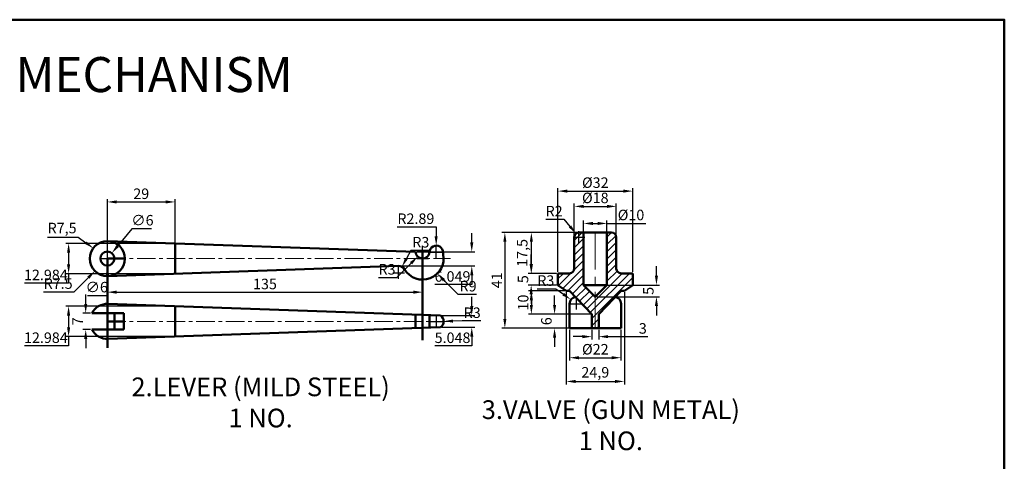
# Model space of a CAD drawing. Units: millimetres. Extents: x -166 to 681, y -4360 to 126.
# Tile 7 of 7: x 259 to 681, y -63 to 126. Entities that reach past the tile are written whole.
import ezdxf

# ---------------------------------------------------------------- set-up
doc = ezdxf.new("R2010")
doc.units = ezdxf.units.MM
doc.header["$LTSCALE"] = 0.5
doc.linetypes.add('CENTER', pattern=[50.8, 31.75, -6.35, 6.35, -6.35])
for name, color, linetype, lineweight in [('M-CNTR', 1, 'CENTER', 18), ('M-DIMS', 2, 'Continuous', 25), ('M-HATC', 8, 'Continuous', 18), ('M-OUTL', 7, 'Continuous', 50), ('M-TEXT', 7, 'Continuous', 25), ('M-TTLB', 7, 'Continuous', 50)]:
    doc.layers.add(name, color=color, linetype=linetype, lineweight=lineweight)
doc.styles.get("Standard").update_dxf_attribs({"font": 'arial.ttf'})
doc.dimstyles.new('ISO-25', dxfattribs={"dimtxt": 4.5, "dimasz": 4, "dimexe": 1.25, "dimexo": 0.625, "dimtad": 1, "dimtoh": 1, "dimdec": 1, "dimtxsty": 'Standard', "dimcen": 2.5, "dimadec": 0, "dimazin": 0, "dimtfac": 1, "dimtdec": 1, "dimtofl": 0, "dimtmove": 0, "dimatfit": 3, "dimfxl": 1, "dimarcsym": 0})

# ---------------------------------------------------------------- blocks, each defined once
blk = doc.blocks.new('*D25')
at = {"layer": 'Defpoints', "color": 0, "ltscale": 0.5, "transparency": 16777216}
for p in [(521.63, 52.7), (489.63, 17.51), (521.63, 17.51)]:
    blk.add_point(p, dxfattribs=at)
at = {"layer": 'M-DIMS', "color": 0, "lineweight": -2, "ltscale": 0.5, "transparency": 16777216}
for p, q in [((489.63, 18.13), (489.63, 53.95)), ((493.63, 52.7), (517.63, 52.7)), ((521.63, 18.13), (521.63, 53.95))]:
    blk.add_line(p, q, dxfattribs=at)
at = {"layer": 'M-DIMS', "color": 0, "ltscale": 0.5, "transparency": 16777216}
for points in [[(493.63, 53.37), (493.63, 52.04), (489.63, 52.7)], [(517.63, 53.37), (517.63, 52.04), (521.63, 52.7)]]:
    blk.add_solid(points, dxfattribs=at)
at = {"layer": 'M-DIMS', "color": 0, "ltscale": 0.5, "transparency": 16777216, "insert": (505.63, 55.75), "char_height": 4.5, "attachment_point": 5}
blk.add_mtext('%%C32', dxfattribs=at)
blk = doc.blocks.new('*D26')
at = {"layer": 'Defpoints', "color": 0, "ltscale": 0.5, "transparency": 16777216}
for p in [(510.63, 38.86), (500.63, 35.01), (510.63, 35.01)]:
    blk.add_point(p, dxfattribs=at)
at = {"layer": 'M-DIMS', "color": 0, "lineweight": -2, "ltscale": 0.5, "transparency": 16777216}
for p, q in [((500.63, 35.63), (500.63, 40.11)), ((504.63, 38.86), (506.63, 38.86)), ((510.63, 35.63), (510.63, 40.11)), ((510.63, 38.86), (527.21, 38.86))]:
    blk.add_line(p, q, dxfattribs=at)
at = {"layer": 'M-DIMS', "color": 0, "ltscale": 0.5, "transparency": 16777216}
for points in [[(504.63, 39.53), (504.63, 38.19), (500.63, 38.86)], [(506.63, 39.53), (506.63, 38.19), (510.63, 38.86)]]:
    blk.add_solid(points, dxfattribs=at)
at = {"layer": 'M-DIMS', "color": 0, "ltscale": 0.5, "transparency": 16777216, "insert": (520.92, 41.91), "char_height": 4.5, "attachment_point": 5}
blk.add_mtext('%%C10', dxfattribs=at)
blk = doc.blocks.new('*D27')
at = {"layer": 'Defpoints', "color": 0, "ltscale": 0.5, "transparency": 16777216}
for p in [(514.63, 46.17), (496.63, 26.26), (514.63, 26.26)]:
    blk.add_point(p, dxfattribs=at)
at = {"layer": 'M-DIMS', "color": 0, "lineweight": -2, "ltscale": 0.5, "transparency": 16777216}
for p, q in [((496.63, 26.88), (496.63, 47.42)), ((514.63, 26.88), (514.63, 47.42)), ((500.63, 46.17), (510.63, 46.17))]:
    blk.add_line(p, q, dxfattribs=at)
at = {"layer": 'M-DIMS', "color": 0, "ltscale": 0.5, "transparency": 16777216}
for points in [[(500.63, 46.84), (500.63, 45.51), (496.63, 46.17)], [(510.63, 46.84), (510.63, 45.51), (514.63, 46.17)]]:
    blk.add_solid(points, dxfattribs=at)
at = {"layer": 'M-DIMS', "color": 0, "ltscale": 0.5, "transparency": 16777216, "insert": (505.63, 49.22), "char_height": 4.5, "attachment_point": 5}
blk.add_mtext('%%C18', dxfattribs=at)
blk = doc.blocks.new('*D28')
at = {"layer": 'Defpoints', "color": 0, "ltscale": 0.5, "transparency": 16777216}
for p in [(505.63, 12.51), (505.63, 7.51), (531.82, 7.51)]:
    blk.add_point(p, dxfattribs=at)
at = {"layer": 'M-DIMS', "color": 0, "lineweight": -2, "ltscale": 0.5, "transparency": 16777216}
for p, q in [((531.82, 16.51), (531.82, 20.51)), ((506.26, 12.51), (533.07, 12.51)), ((506.26, 7.51), (533.07, 7.51)), ((531.82, 3.51), (531.82, -0.49))]:
    blk.add_line(p, q, dxfattribs=at)
at = {"layer": 'M-DIMS', "color": 0, "ltscale": 0.5, "transparency": 16777216}
for points in [[(531.15, 16.51), (532.49, 16.51), (531.82, 12.51)], [(531.15, 3.51), (532.49, 3.51), (531.82, 7.51)]]:
    blk.add_solid(points, dxfattribs=at)
at = {"layer": 'M-DIMS', "color": 0, "ltscale": 0.5, "transparency": 16777216, "insert": (528.91, 10.01), "char_height": 4.5, "attachment_point": 5, "rotation": 90}
blk.add_mtext('5', dxfattribs=at)
blk = doc.blocks.new('*D29')
at = {"layer": 'Defpoints', "color": 0, "ltscale": 0.5, "transparency": 16777216}
for p in [(505.63, 35.01), (466.89, -5.99), (505.63, -5.99)]:
    blk.add_point(p, dxfattribs=at)
at = {"layer": 'M-DIMS', "color": 0, "lineweight": -2, "ltscale": 0.5, "transparency": 16777216}
for p, q in [((505.01, 35.01), (465.64, 35.01)), ((466.89, 31.01), (466.89, -1.99)), ((505.01, -5.99), (465.64, -5.99))]:
    blk.add_line(p, q, dxfattribs=at)
at = {"layer": 'M-DIMS', "color": 0, "ltscale": 0.5, "transparency": 16777216}
for points in [[(466.23, 31.01), (467.56, 31.01), (466.89, 35.01)], [(466.23, -1.99), (467.56, -1.99), (466.89, -5.99)]]:
    blk.add_solid(points, dxfattribs=at)
at = {"layer": 'M-DIMS', "color": 0, "ltscale": 0.5, "transparency": 16777216, "insert": (464.01, 14.51), "char_height": 4.5, "attachment_point": 5, "rotation": 90}
blk.add_mtext('41', dxfattribs=at)
blk = doc.blocks.new('*D30')
at = {"layer": 'Defpoints', "color": 0, "ltscale": 0.5, "transparency": 16777216}
for p in [(478.25, 35.01), (485.33, 35.01), (489.63, 17.51)]:
    blk.add_point(p, dxfattribs=at)
at = {"layer": 'M-DIMS', "color": 0, "lineweight": -2, "ltscale": 0.5, "transparency": 16777216}
for p, q in [((484.7, 35.01), (477, 35.01)), ((478.25, 21.51), (478.25, 31.01)), ((489.01, 17.51), (477, 17.51))]:
    blk.add_line(p, q, dxfattribs=at)
at = {"layer": 'M-DIMS', "color": 0, "ltscale": 0.5, "transparency": 16777216}
for points in [[(477.58, 31.01), (478.91, 31.01), (478.25, 35.01)], [(477.58, 21.51), (478.91, 21.51), (478.25, 17.51)]]:
    blk.add_solid(points, dxfattribs=at)
at = {"layer": 'M-DIMS', "color": 0, "ltscale": 0.5, "transparency": 16777216, "insert": (474.92, 26.26), "char_height": 4.5, "attachment_point": 5, "rotation": 90}
blk.add_mtext('17,5', dxfattribs=at)
blk = doc.blocks.new('*D31')
at = {"layer": 'Defpoints', "color": 0, "ltscale": 0.5, "transparency": 16777216}
for p in [(493.19, 10.01), (478.25, 0.01), (504.13, 0.01)]:
    blk.add_point(p, dxfattribs=at)
at = {"layer": 'M-DIMS', "color": 0, "lineweight": -2, "ltscale": 0.5, "transparency": 16777216}
for p, q in [((492.57, 10.01), (477, 10.01)), ((478.25, 6.01), (478.25, 4.01)), ((503.51, 0.01), (477, 0.01))]:
    blk.add_line(p, q, dxfattribs=at)
at = {"layer": 'M-DIMS', "color": 0, "ltscale": 0.5, "transparency": 16777216}
for points in [[(477.58, 6.01), (478.91, 6.01), (478.25, 10.01)], [(477.58, 4.01), (478.91, 4.01), (478.25, 0.01)]]:
    blk.add_solid(points, dxfattribs=at)
at = {"layer": 'M-DIMS', "color": 0, "ltscale": 0.5, "transparency": 16777216, "insert": (475.32, 5.01), "char_height": 4.5, "attachment_point": 5, "rotation": 90}
blk.add_mtext('10', dxfattribs=at)
blk = doc.blocks.new('*D32')
at = {"layer": 'Defpoints', "color": 0, "ltscale": 0.5, "transparency": 16777216}
for p in [(504.13, 0.01), (488.18, -5.99), (504.13, -5.99)]:
    blk.add_point(p, dxfattribs=at)
at = {"layer": 'M-DIMS', "color": 0, "lineweight": -2, "ltscale": 0.5, "transparency": 16777216}
for p, q in [((488.18, 4.01), (488.18, 8.01)), ((503.51, 0.01), (486.93, 0.01)), ((503.51, -5.99), (486.93, -5.99)), ((488.18, -9.99), (488.18, -13.99))]:
    blk.add_line(p, q, dxfattribs=at)
at = {"layer": 'M-DIMS', "color": 0, "ltscale": 0.5, "transparency": 16777216}
for points in [[(487.52, 4.01), (488.85, 4.01), (488.18, 0.01)], [(487.52, -9.99), (488.85, -9.99), (488.18, -5.99)]]:
    blk.add_solid(points, dxfattribs=at)
at = {"layer": 'M-DIMS', "color": 0, "ltscale": 0.5, "transparency": 16777216, "insert": (485.26, -2.99), "char_height": 4.5, "attachment_point": 5, "rotation": 90}
blk.add_mtext('6', dxfattribs=at)
blk = doc.blocks.new('*D33')
at = {"layer": 'Defpoints', "color": 0, "ltscale": 0.5, "transparency": 16777216}
for p in [(489.63, 17.51), (478.15, 12.51), (489.63, 12.51)]:
    blk.add_point(p, dxfattribs=at)
at = {"layer": 'M-DIMS', "color": 0, "lineweight": -2, "ltscale": 0.5, "transparency": 16777216}
for p, q in [((478.15, 21.51), (478.15, 25.51)), ((489.01, 17.51), (476.9, 17.51)), ((489.01, 12.51), (476.9, 12.51)), ((478.15, 8.51), (478.15, 4.51))]:
    blk.add_line(p, q, dxfattribs=at)
at = {"layer": 'M-DIMS', "color": 0, "ltscale": 0.5, "transparency": 16777216}
for points in [[(477.48, 21.51), (478.82, 21.51), (478.15, 17.51)], [(477.48, 8.51), (478.82, 8.51), (478.15, 12.51)]]:
    blk.add_solid(points, dxfattribs=at)
at = {"layer": 'M-DIMS', "color": 0, "ltscale": 0.5, "transparency": 16777216, "insert": (475.24, 15.01), "char_height": 4.5, "attachment_point": 5, "rotation": 90}
blk.add_mtext('5', dxfattribs=at)
blk = doc.blocks.new('*D34')
at = {"layer": 'Defpoints', "color": 0, "ltscale": 0.5, "transparency": 16777216}
for p in [(504.13, -5.99), (507.13, -5.99), (507.13, -9.59)]:
    blk.add_point(p, dxfattribs=at)
at = {"layer": 'M-DIMS', "color": 0, "lineweight": -2, "ltscale": 0.5, "transparency": 16777216}
for p, q in [((504.13, -6.62), (504.13, -10.84)), ((507.13, -6.62), (507.13, -10.84)), ((500.13, -9.59), (496.13, -9.59)), ((511.13, -9.59), (528.08, -9.59))]:
    blk.add_line(p, q, dxfattribs=at)
at = {"layer": 'M-DIMS', "color": 0, "ltscale": 0.5, "transparency": 16777216}
for points in [[(500.13, -8.92), (500.13, -10.25), (504.13, -9.59)], [(511.13, -8.92), (511.13, -10.25), (507.13, -9.59)]]:
    blk.add_solid(points, dxfattribs=at)
at = {"layer": 'M-DIMS', "color": 0, "ltscale": 0.5, "transparency": 16777216, "insert": (525.98, -6.66), "char_height": 4.5, "attachment_point": 5}
blk.add_mtext('3', dxfattribs=at)
blk = doc.blocks.new('*D35')
at = {"layer": 'Defpoints', "color": 0, "ltscale": 0.5, "transparency": 16777216}
for p in [(494.63, -5.99), (516.63, -5.99), (516.63, -18.62)]:
    blk.add_point(p, dxfattribs=at)
at = {"layer": 'M-DIMS', "color": 0, "lineweight": -2, "ltscale": 0.5, "transparency": 16777216}
for p, q in [((494.63, -6.62), (494.63, -19.87)), ((516.63, -6.62), (516.63, -19.87)), ((498.63, -18.62), (512.63, -18.62))]:
    blk.add_line(p, q, dxfattribs=at)
at = {"layer": 'M-DIMS', "color": 0, "ltscale": 0.5, "transparency": 16777216}
for points in [[(498.63, -17.95), (498.63, -19.29), (494.63, -18.62)], [(512.63, -17.95), (512.63, -19.29), (516.63, -18.62)]]:
    blk.add_solid(points, dxfattribs=at)
at = {"layer": 'M-DIMS', "color": 0, "ltscale": 0.5, "transparency": 16777216, "insert": (505.63, -15.57), "char_height": 4.5, "attachment_point": 5}
blk.add_mtext('%%C22', dxfattribs=at)
blk = doc.blocks.new('*D36')
at = {"layer": 'Defpoints', "color": 0, "ltscale": 0.5, "transparency": 16777216}
for p in [(493.19, 10.01), (518.08, 10.01), (518.08, -28.77)]:
    blk.add_point(p, dxfattribs=at)
at = {"layer": 'M-DIMS', "color": 0, "lineweight": -2, "ltscale": 0.5, "transparency": 16777216}
for p, q in [((493.19, 9.38), (493.19, -30.02)), ((518.08, 9.38), (518.08, -30.02)), ((497.19, -28.77), (514.08, -28.77))]:
    blk.add_line(p, q, dxfattribs=at)
at = {"layer": 'M-DIMS', "color": 0, "ltscale": 0.5, "transparency": 16777216}
for points in [[(497.19, -28.11), (497.19, -29.44), (493.19, -28.77)], [(514.08, -28.11), (514.08, -29.44), (518.08, -28.77)]]:
    blk.add_solid(points, dxfattribs=at)
at = {"layer": 'M-DIMS', "color": 0, "ltscale": 0.5, "transparency": 16777216, "insert": (505.63, -25.44), "char_height": 4.5, "attachment_point": 5}
blk.add_mtext('24,9', dxfattribs=at)
blk = doc.blocks.new('*D69')
at = {"layer": 'Defpoints', "color": 0, "ltscale": 0.5, "transparency": 16777216}
for p in [(298.56, 26.14), (294.76, 21.5)]:
    blk.add_point(p, dxfattribs=at)
at = {"layer": 'M-DIMS', "color": 0, "lineweight": -2, "ltscale": 0.5, "transparency": 16777216}
for p, q in [((307.13, 36.61), (301.1, 29.24)), ((315.6, 36.61), (307.13, 36.61)), ((296.66, 21.32), (296.66, 26.32)), ((294.16, 23.82), (299.16, 23.82))]:
    blk.add_line(p, q, dxfattribs=at)
at = {"layer": 'M-DIMS', "color": 0, "ltscale": 0.5, "transparency": 16777216}
blk.add_solid([(300.58, 29.66), (301.61, 28.82), (298.56, 26.14)], dxfattribs=at)
at = {"layer": 'M-DIMS', "color": 0, "ltscale": 0.5, "transparency": 16777216, "insert": (311.68, 39.66), "char_height": 4.5, "attachment_point": 5}
blk.add_mtext('∅6', dxfattribs=at)
blk = doc.blocks.new('*D70')
at = {"layer": 'Defpoints', "color": 0, "ltscale": 0.5, "transparency": 16777216}
for p in [(290.61, 28.26), (296.66, 23.82)]:
    blk.add_point(p, dxfattribs=at)
at = {"layer": 'M-DIMS', "color": 0, "lineweight": -2, "ltscale": 0.5, "transparency": 16777216}
for p, q in [((271.01, 33), (284.17, 33)), ((284.17, 33), (287.39, 30.63)), ((296.66, 21.32), (296.66, 26.32)), ((294.16, 23.82), (299.16, 23.82))]:
    blk.add_line(p, q, dxfattribs=at)
at = {"layer": 'M-DIMS', "color": 0, "ltscale": 0.5, "transparency": 16777216}
blk.add_solid([(287.78, 31.17), (287, 30.09), (290.61, 28.26)], dxfattribs=at)
at = {"layer": 'M-DIMS', "color": 0, "ltscale": 0.5, "transparency": 16777216, "insert": (277.27, 36.32), "char_height": 4.5, "attachment_point": 5}
blk.add_mtext('R7,5', dxfattribs=at)
blk = doc.blocks.new('*D71')
at = {"layer": 'Defpoints', "color": 0, "ltscale": 0.5, "transparency": 16777216}
for p in [(325.66, 48.07), (296.66, 23.82), (325.66, 23.82)]:
    blk.add_point(p, dxfattribs=at)
at = {"layer": 'M-DIMS', "color": 0, "lineweight": -2, "ltscale": 0.5, "transparency": 16777216}
for p, q in [((296.66, 24.45), (296.66, 49.32)), ((300.66, 48.07), (321.66, 48.07)), ((325.66, 24.45), (325.66, 49.32))]:
    blk.add_line(p, q, dxfattribs=at)
at = {"layer": 'M-DIMS', "color": 0, "ltscale": 0.5, "transparency": 16777216}
for points in [[(300.66, 48.74), (300.66, 47.4), (296.66, 48.07)], [(321.66, 48.74), (321.66, 47.4), (325.66, 48.07)]]:
    blk.add_solid(points, dxfattribs=at)
at = {"layer": 'M-DIMS', "color": 0, "ltscale": 0.5, "transparency": 16777216, "insert": (311.16, 50.99), "char_height": 4.5, "attachment_point": 5}
blk.add_mtext('29', dxfattribs=at)
blk = doc.blocks.new('*D72')
at = {"layer": 'Defpoints', "color": 0, "ltscale": 0.5, "transparency": 16777216}
for p in [(296.66, 10.75), (431.66, 10.75), (431.66, 9.45)]:
    blk.add_point(p, dxfattribs=at)
at = {"layer": 'M-DIMS', "color": 0, "lineweight": -2, "ltscale": 0.5, "transparency": 16777216}
for p, q in [((296.66, 10.12), (296.66, 8.2)), ((300.66, 9.45), (427.66, 9.45)), ((431.66, 10.12), (431.66, 8.2))]:
    blk.add_line(p, q, dxfattribs=at)
at = {"layer": 'M-DIMS', "color": 0, "ltscale": 0.5, "transparency": 16777216}
for points in [[(300.66, 10.12), (300.66, 8.79), (296.66, 9.45)], [(427.66, 10.12), (427.66, 8.79), (431.66, 9.45)]]:
    blk.add_solid(points, dxfattribs=at)
at = {"layer": 'M-DIMS', "color": 0, "ltscale": 0.5, "transparency": 16777216, "insert": (364.16, 12.38), "char_height": 4.5, "attachment_point": 5}
blk.add_mtext('135', dxfattribs=at)
blk = doc.blocks.new('*D73')
at = {"layer": 'Defpoints', "color": 0, "ltscale": 0.5, "transparency": 16777216}
for p in [(290.03, 0.45), (287.39, -6.55), (290.03, -6.55)]:
    blk.add_point(p, dxfattribs=at)
at = {"layer": 'M-DIMS', "color": 0, "lineweight": -2, "ltscale": 0.5, "transparency": 16777216}
for p, q in [((287.39, 4.45), (287.39, 8.45)), ((289.4, 0.45), (286.14, 0.45)), ((289.4, -6.55), (286.14, -6.55)), ((287.39, -10.55), (287.39, -14.55))]:
    blk.add_line(p, q, dxfattribs=at)
at = {"layer": 'M-DIMS', "color": 0, "ltscale": 0.5, "transparency": 16777216}
for points in [[(286.72, 4.45), (288.05, 4.45), (287.39, 0.45)], [(286.72, -10.55), (288.05, -10.55), (287.39, -6.55)]]:
    blk.add_solid(points, dxfattribs=at)
at = {"layer": 'M-DIMS', "color": 0, "ltscale": 0.5, "transparency": 16777216, "insert": (284.51, -3.05), "char_height": 4.5, "attachment_point": 5, "rotation": 90}
blk.add_mtext('7', dxfattribs=at)
blk = doc.blocks.new('*D83')
at = {"layer": 'Defpoints', "color": 0, "ltscale": 0.5, "transparency": 16777216}
for p in [(325.66, 30.32), (280.06, 17.33), (325.66, 17.33)]:
    blk.add_point(p, dxfattribs=at)
at = {"layer": 'M-DIMS', "color": 0, "lineweight": -2, "ltscale": 0.5, "transparency": 16777216}
for p, q in [((325.04, 30.32), (278.81, 30.32)), ((280.06, 26.32), (280.06, 21.33)), ((325.04, 17.33), (278.81, 17.33)), ((280.06, 17.33), (280.06, 13.33)), ((280.06, 13.33), (261.2, 13.33))]:
    blk.add_line(p, q, dxfattribs=at)
at = {"layer": 'M-DIMS', "color": 0, "ltscale": 0.5, "transparency": 16777216}
for points in [[(279.39, 26.32), (280.73, 26.32), (280.06, 30.32)], [(279.39, 21.33), (280.73, 21.33), (280.06, 17.33)]]:
    blk.add_solid(points, dxfattribs=at)
at = {"layer": 'M-DIMS', "color": 0, "ltscale": 0.5, "transparency": 16777216, "insert": (270.32, 16.25), "char_height": 4.5, "attachment_point": 5}
blk.add_mtext('12.984', dxfattribs=at)
blk = doc.blocks.new('*D84')
at = {"layer": 'Defpoints', "color": 0, "ltscale": 0.5, "transparency": 16777216}
for p in [(428.66, 26.72), (421.25, 20.67), (452.72, 20.67)]:
    blk.add_point(p, dxfattribs=at)
at = {"layer": 'M-DIMS', "color": 0, "lineweight": -2, "ltscale": 0.5, "transparency": 16777216}
for p, q in [((452.72, 30.72), (452.72, 34.72)), ((429.29, 26.72), (453.97, 26.72)), ((421.88, 20.67), (453.97, 20.67)), ((452.72, 12.67), (436.87, 12.67)), ((452.72, 16.67), (452.72, 12.67))]:
    blk.add_line(p, q, dxfattribs=at)
at = {"layer": 'M-DIMS', "color": 0, "ltscale": 0.5, "transparency": 16777216}
for points in [[(452.05, 30.72), (453.38, 30.72), (452.72, 26.72)], [(452.05, 16.67), (453.38, 16.67), (452.72, 20.67)]]:
    blk.add_solid(points, dxfattribs=at)
at = {"layer": 'M-DIMS', "color": 0, "ltscale": 0.5, "transparency": 16777216, "insert": (444.48, 15.59), "char_height": 4.5, "attachment_point": 5}
blk.add_mtext('6.049', dxfattribs=at)
blk = doc.blocks.new('*D85')
at = {"layer": 'Defpoints', "color": 0, "ltscale": 0.5, "transparency": 16777216}
for p in [(439.28, -0.53), (439.28, -5.58), (452.72, -5.58)]:
    blk.add_point(p, dxfattribs=at)
at = {"layer": 'M-DIMS', "color": 0, "lineweight": -2, "ltscale": 0.5, "transparency": 16777216}
for p, q in [((452.72, 3.47), (452.72, 7.47)), ((439.91, -0.53), (453.97, -0.53)), ((439.91, -5.58), (453.97, -5.58)), ((452.72, -9.58), (452.72, -13.58)), ((452.72, -13.58), (436.9, -13.58))]:
    blk.add_line(p, q, dxfattribs=at)
at = {"layer": 'M-DIMS', "color": 0, "ltscale": 0.5, "transparency": 16777216}
for points in [[(452.05, 3.47), (453.38, 3.47), (452.72, -0.53)], [(452.05, -9.58), (453.38, -9.58), (452.72, -5.58)]]:
    blk.add_solid(points, dxfattribs=at)
at = {"layer": 'M-DIMS', "color": 0, "ltscale": 0.5, "transparency": 16777216, "insert": (444.49, -10.65), "char_height": 4.5, "attachment_point": 5}
blk.add_mtext('5.048', dxfattribs=at)
blk = doc.blocks.new('*D86')
at = {"layer": 'Defpoints', "color": 0, "ltscale": 0.5, "transparency": 16777216}
for p in [(325.66, 3.44), (280.06, -9.54), (325.66, -9.54)]:
    blk.add_point(p, dxfattribs=at)
at = {"layer": 'M-DIMS', "color": 0, "lineweight": -2, "ltscale": 0.5, "transparency": 16777216}
for p, q in [((325.04, 3.44), (278.81, 3.44)), ((280.06, -0.56), (280.06, -5.54)), ((325.04, -9.54), (278.81, -9.54)), ((280.06, -9.54), (280.06, -13.54)), ((280.06, -13.54), (261.2, -13.54))]:
    blk.add_line(p, q, dxfattribs=at)
at = {"layer": 'M-DIMS', "color": 0, "ltscale": 0.5, "transparency": 16777216}
for points in [[(279.39, -0.56), (280.73, -0.56), (280.06, 3.44)], [(279.39, -5.54), (280.73, -5.54), (280.06, -9.54)]]:
    blk.add_solid(points, dxfattribs=at)
at = {"layer": 'M-DIMS', "color": 0, "ltscale": 0.5, "transparency": 16777216, "insert": (270.32, -10.62), "char_height": 4.5, "attachment_point": 5}
blk.add_mtext('12.984', dxfattribs=at)
blk = doc.blocks.new('*D94')
at = {"layer": 'Defpoints', "color": 0, "ltscale": 0.5, "transparency": 16777216}
for p in [(296.66, 23.82), (291.36, 18.52)]:
    blk.add_point(p, dxfattribs=at)
at = {"layer": 'M-DIMS', "color": 0, "lineweight": -2, "ltscale": 0.5, "transparency": 16777216}
for p, q in [((296.66, 21.32), (296.66, 26.32)), ((294.16, 23.82), (299.16, 23.82)), ((282.47, 9.62), (288.53, 15.69)), ((269.31, 9.62), (282.47, 9.62))]:
    blk.add_line(p, q, dxfattribs=at)
at = {"layer": 'M-DIMS', "color": 0, "ltscale": 0.5, "transparency": 16777216}
blk.add_solid([(288.06, 16.16), (289, 15.22), (291.36, 18.52)], dxfattribs=at)
at = {"layer": 'M-DIMS', "color": 0, "ltscale": 0.5, "transparency": 16777216, "insert": (275.58, 12.54), "char_height": 4.5, "attachment_point": 5}
blk.add_mtext('R7.5', dxfattribs=at)
blk = doc.blocks.new('*D95')
at = {"layer": 'Defpoints', "color": 0, "ltscale": 0.5, "transparency": 16777216}
for p in [(296.66, 26.82), (296.66, 20.82)]:
    blk.add_point(p, dxfattribs=at)
at = {"layer": 'M-DIMS', "color": 0, "lineweight": -2, "ltscale": 0.5, "transparency": 16777216}
for p, q in [((296.66, 21.32), (296.66, 26.32)), ((294.16, 23.82), (299.16, 23.82)), ((296.66, 7.98), (296.66, 16.82)), ((288.19, 7.98), (296.66, 7.98))]:
    blk.add_line(p, q, dxfattribs=at)
at = {"layer": 'M-DIMS', "color": 0, "ltscale": 0.5, "transparency": 16777216}
blk.add_solid([(295.99, 16.82), (297.33, 16.82), (296.66, 20.82)], dxfattribs=at)
at = {"layer": 'M-DIMS', "color": 0, "ltscale": 0.5, "transparency": 16777216, "insert": (292.11, 11.03), "char_height": 4.5, "attachment_point": 5}
blk.add_mtext('∅6', dxfattribs=at)
blk = doc.blocks.new('*D96')
at = {"layer": 'Defpoints', "color": 0, "ltscale": 0.5, "transparency": 16777216}
for p in [(431.66, 26.82), (429.55, 24.69)]:
    blk.add_point(p, dxfattribs=at)
at = {"layer": 'M-DIMS', "color": 0, "lineweight": -2, "ltscale": 0.5, "transparency": 16777216}
for p, q in [((429.16, 26.82), (434.16, 26.82)), ((431.66, 24.32), (431.66, 29.32)), ((420.69, 15.74), (426.74, 21.85)), ((412.81, 15.74), (420.69, 15.74))]:
    blk.add_line(p, q, dxfattribs=at)
at = {"layer": 'M-DIMS', "color": 0, "ltscale": 0.5, "transparency": 16777216}
blk.add_solid([(426.26, 22.32), (427.21, 21.38), (429.55, 24.69)], dxfattribs=at)
at = {"layer": 'M-DIMS', "color": 0, "ltscale": 0.5, "transparency": 16777216, "insert": (416.44, 18.66), "char_height": 4.5, "attachment_point": 5}
blk.add_mtext('R3', dxfattribs=at)
blk = doc.blocks.new('*D97')
at = {"layer": 'Defpoints', "color": 0, "ltscale": 0.5, "transparency": 16777216}
for p in [(437.5, 29.4), (437.53, 26.51)]:
    blk.add_point(p, dxfattribs=at)
at = {"layer": 'M-DIMS', "color": 0, "lineweight": -2, "ltscale": 0.5, "transparency": 16777216}
for p, q in [((420.78, 37.4), (437.41, 37.4)), ((437.41, 37.4), (437.45, 33.4)), ((435.03, 26.51), (440.03, 26.51)), ((437.53, 24.01), (437.53, 29.01))]:
    blk.add_line(p, q, dxfattribs=at)
at = {"layer": 'M-DIMS', "color": 0, "ltscale": 0.5, "transparency": 16777216}
blk.add_solid([(438.12, 33.41), (436.79, 33.39), (437.5, 29.4)], dxfattribs=at)
at = {"layer": 'M-DIMS', "color": 0, "ltscale": 0.5, "transparency": 16777216, "insert": (428.78, 40.32), "char_height": 4.5, "attachment_point": 5}
blk.add_mtext('R2.89', dxfattribs=at)
blk = doc.blocks.new('*D98')
at = {"layer": 'Defpoints', "color": 0, "ltscale": 0.5, "transparency": 16777216}
for p in [(431.66, 23.82), (438, 17.44)]:
    blk.add_point(p, dxfattribs=at)
at = {"layer": 'M-DIMS', "color": 0, "lineweight": -2, "ltscale": 0.5, "transparency": 16777216}
for p, q in [((431.66, 21.32), (431.66, 26.32)), ((429.16, 23.82), (434.16, 23.82)), ((446.88, 8.5), (440.82, 14.6)), ((454.77, 8.5), (446.88, 8.5))]:
    blk.add_line(p, q, dxfattribs=at)
at = {"layer": 'M-DIMS', "color": 0, "ltscale": 0.5, "transparency": 16777216}
blk.add_solid([(441.29, 15.07), (440.35, 14.13), (438, 17.44)], dxfattribs=at)
at = {"layer": 'M-DIMS', "color": 0, "ltscale": 0.5, "transparency": 16777216, "insert": (451.14, 11.42), "char_height": 4.5, "attachment_point": 5}
blk.add_mtext('R9', dxfattribs=at)
blk = doc.blocks.new('*D99')
at = {"layer": 'Defpoints', "color": 0, "ltscale": 0.5, "transparency": 16777216}
for p in [(421.36, 17.67), (422.8, 20.3)]:
    blk.add_point(p, dxfattribs=at)
at = {"layer": 'M-DIMS', "color": 0, "lineweight": -2, "ltscale": 0.5, "transparency": 16777216}
for p, q in [((426.65, 27.31), (424.73, 23.81)), ((434.53, 27.31), (426.65, 27.31)), ((418.86, 17.67), (423.86, 17.67)), ((421.36, 15.17), (421.36, 20.17))]:
    blk.add_line(p, q, dxfattribs=at)
at = {"layer": 'M-DIMS', "color": 0, "ltscale": 0.5, "transparency": 16777216}
blk.add_solid([(424.14, 24.13), (425.31, 23.49), (422.8, 20.3)], dxfattribs=at)
at = {"layer": 'M-DIMS', "color": 0, "ltscale": 0.5, "transparency": 16777216, "insert": (430.9, 30.24), "char_height": 4.5, "attachment_point": 5}
blk.add_mtext('R3', dxfattribs=at)
blk = doc.blocks.new('*D100')
at = {"layer": 'Defpoints', "color": 0, "ltscale": 0.5, "transparency": 16777216}
for p in [(437.66, -3.05), (440.66, -3)]:
    blk.add_point(p, dxfattribs=at)
at = {"layer": 'M-DIMS', "color": 0, "lineweight": -2, "ltscale": 0.5, "transparency": 16777216}
for p, q in [((435.16, -3.05), (440.16, -3.05)), ((437.66, -5.55), (437.66, -0.55)), ((448.66, -2.85), (444.66, -2.93)), ((456.54, -2.85), (448.66, -2.85))]:
    blk.add_line(p, q, dxfattribs=at)
at = {"layer": 'M-DIMS', "color": 0, "ltscale": 0.5, "transparency": 16777216}
blk.add_solid([(444.65, -2.26), (444.67, -3.59), (440.66, -3)], dxfattribs=at)
at = {"layer": 'M-DIMS', "color": 0, "ltscale": 0.5, "transparency": 16777216, "insert": (452.91, 0.07), "char_height": 4.5, "attachment_point": 5}
blk.add_mtext('R3', dxfattribs=at)
blk = doc.blocks.new('*D101')
at = {"layer": 'Defpoints', "color": 0, "ltscale": 0.5, "transparency": 16777216}
for p in [(497.35, 34.54), (498.63, 33.01)]:
    blk.add_point(p, dxfattribs=at)
at = {"layer": 'M-DIMS', "color": 0, "lineweight": -2, "ltscale": 0.5, "transparency": 16777216}
for p, q in [((484.38, 40.68), (492.22, 40.68)), ((492.22, 40.68), (494.78, 37.61)), ((498.63, 30.51), (498.63, 35.51)), ((496.13, 33.01), (501.13, 33.01))]:
    blk.add_line(p, q, dxfattribs=at)
at = {"layer": 'M-DIMS', "color": 0, "ltscale": 0.5, "transparency": 16777216}
blk.add_solid([(495.29, 38.04), (494.27, 37.18), (497.35, 34.54)], dxfattribs=at)
at = {"layer": 'M-DIMS', "color": 0, "ltscale": 0.5, "transparency": 16777216, "insert": (487.99, 43.56), "char_height": 4.5, "attachment_point": 5}
blk.add_mtext('R2', dxfattribs=at)
blk = doc.blocks.new('*D102')
at = {"layer": 'Defpoints', "color": 0, "ltscale": 0.5, "transparency": 16777216}
for p in [(495.19, 6.25), (497.63, 4.51)]:
    blk.add_point(p, dxfattribs=at)
at = {"layer": 'M-DIMS', "color": 0, "lineweight": -2, "ltscale": 0.5, "transparency": 16777216}
for p, q in [((480.8, 10.9), (488.68, 10.9)), ((488.68, 10.9), (491.94, 8.57)), ((495.13, 4.51), (500.13, 4.51)), ((497.63, 2.01), (497.63, 7.01))]:
    blk.add_line(p, q, dxfattribs=at)
at = {"layer": 'M-DIMS', "color": 0, "ltscale": 0.5, "transparency": 16777216}
blk.add_solid([(492.32, 9.12), (491.55, 8.03), (495.19, 6.25)], dxfattribs=at)
at = {"layer": 'M-DIMS', "color": 0, "ltscale": 0.5, "transparency": 16777216, "insert": (484.43, 13.82), "char_height": 4.5, "attachment_point": 5}
blk.add_mtext('R3', dxfattribs=at)

msp = doc.modelspace()

# ---------------------------------------------------------------- hatches: boundary and pattern name
at = {"layer": 'M-HATC', "ltscale": 0.5}
h = msp.add_hatch(dxfattribs=at)
h.set_pattern_fill('ANSI31', color=256, scale=0.7)
h.set_pattern_definition([(45, (-557903.1008, -289970.2781), (-1.571544821, 1.571544821), [])])
h.paths.add_polyline_path([(496.6337, 19.5065, -0.41421356), (494.6337, 17.5065), (489.6337, 17.5065), (489.6337, 12.5065), (493.1908, 10.0065), (494.6337, 10.0065), (504.1337, 0.0065), (504.1337, -5.9935), (505.6337, -5.9935), (505.6337, 7.5065), (500.6337, 12.5065), (500.6337, 35.0065), (498.6337, 35.0065, 0.41421356), (496.6337, 33.0065)])
h.paths.add_polyline_path([(514.6337, 33.0065, 0.41421356), (512.6337, 35.0065), (510.6337, 35.0065), (510.6337, 12.5065), (505.6337, 7.5065), (505.6337, -5.9935), (507.1337, -5.9935), (507.1337, 0.0065), (516.6337, 10.0065), (518.0765, 10.0065), (521.6337, 12.5065), (521.6337, 17.5065), (516.6337, 17.5065, -0.41421356), (514.6337, 19.5065)])

# ---------------------------------------------------------------- linework, layer by layer
at = {"layer": 'M-CNTR'}
for p, q in [((505.6337, 35.0065), (505.6337, 7.5065)), ((505.6337, 7.5065), (505.6337, -5.9935))]:
    msp.add_line(p, q, dxfattribs=at)
at = {"layer": 'M-CNTR', "ltscale": 0.5}
for p, q in [((296.6607, 23.8235), (443.6153, 23.8235)), ((296.6607, -3.053), (443.6153, -3.053))]:
    msp.add_line(p, q, dxfattribs=at)
at = {"layer": 'M-OUTL'}
for p, q in [((498.6337, 35.0065), (512.6337, 35.0065)), ((500.6337, 35.0065), (500.6337, 12.5065)), ((510.6337, 35.0065), (510.6337, 12.5065)), ((496.6337, 33.0065), (496.6337, 19.5065)), ((514.6337, 33.0065), (514.6337, 19.5065)), ((489.6337, 17.5065), (489.6337, 12.5065)), ((494.6337, 17.5065), (489.6337, 17.5065)), ((516.6337, 17.5065), (521.6337, 17.5065)), ((521.6337, 17.5065), (516.6337, 17.5065)), ((521.6337, 12.5065), (521.6337, 17.5065)), ((493.1908, 10.0065), (489.6337, 12.5065)), ((494.6337, 10.0065), (493.1908, 10.0065)), ((504.1337, 0.0065), (494.6337, 10.0065)), ((500.6337, 12.5065), (510.6337, 12.5065)), ((505.6337, 7.5065), (500.6337, 12.5065)), ((505.6337, 7.5065), (510.6337, 12.5065)), ((507.1337, 0.0065), (516.6337, 10.0065)), ((516.6337, 10.0065), (518.0765, 10.0065)), ((518.0765, 10.0065), (521.6337, 12.5065)), ((494.6337, 4.5065), (494.6337, -5.9935)), ((516.6337, 4.5065), (516.6337, -5.9935)), ((504.1337, 0.0065), (504.1337, -5.9935)), ((507.1337, 0.0065), (507.1337, -5.9935)), ((494.6337, -5.9935), (504.1337, -5.9935)), ((504.1337, -5.9935), (516.6337, -5.9935))]:
    msp.add_line(p, q, dxfattribs=at)
at = {"layer": 'M-OUTL', "ltscale": 0.5}
for p, q in [((296.9225, 31.319), (428.6626, 26.7185)), ((325.6607, 17.3317), (325.6607, 30.3154)), ((431.6607, -11.037), (431.6607, 26.8235)), ((296.6607, 23.8235), (304.1607, 23.8235)), ((296.6607, 23.8235), (296.6607, -14.4115)), ((296.9225, 16.3281), (421.2529, 20.6698)), ((296.9225, 4.4425), (439.2821, -0.5288)), ((290.0275, 0.447), (303.6607, 0.447)), ((299.6607, 0.447), (299.6607, -6.553)), ((303.6607, 0.447), (303.6607, -6.553)), ((325.6607, -9.5448), (325.6607, 3.4389)), ((296.6607, -3.053), (304.1607, -3.053)), ((428.6607, -0.2627), (428.6607, -5.8432)), ((434.6607, -0.2627), (434.6607, -5.8432)), ((303.6607, -6.553), (290.0275, -6.553)), ((296.9225, -10.5484), (439.2821, -5.5771))]:
    msp.add_line(p, q, dxfattribs=at)
for radius in [7.5, 3]:
    msp.add_circle((296.6607, 23.8235), radius, dxfattribs=at)
at = {"layer": 'M-OUTL'}
for centre, radius, start, end in [((498.6337, 33.0065), 2, 90, 180), ((512.6337, 33.0065), 2, 0, 90), ((494.6337, 19.5065), 2, 270, 0), ((516.6337, 19.5065), 2, 180, 270), ((497.6337, 4.5065), 3, 101.003457, 180), ((513.6337, 4.5065), 3, 0, 78.996543)]:
    msp.add_arc(centre, radius, start, end, dxfattribs=at)
at = {"layer": 'M-OUTL', "ltscale": 0.5}
for centre, radius, start, end in [((431.6607, 23.8235), 9, 210.841003, 11.557628), ((431.6607, 26.8235), 3, 182.006416, 353.993584), ((437.5342, 26.5096), 2.89, 357.2573, 180), ((443.4174, 26.2278), 3, 177.2573, 191.557628), ((421.3576, 17.6716), 3, 30.841003, 92), ((296.6607, -3.053), 7.5, 88, 152.181861), ((437.6607, -3.053), 3, 302.714431, 57.285569), ((296.6607, -3.053), 7.5, 207.818139, 272)]:
    msp.add_arc(centre, radius, start, end, dxfattribs=at)
at = {"layer": 'M-TTLB', "ltscale": 0.5}
msp.add_lwpolyline([(-165.9437, 126.0872), (680.7907, 126.0872), (680.7907, -430.0081), (-165.9437, -430.0081)], close=True, dxfattribs=at)

# ---------------------------------------------------------------- texts
at = {"layer": 'M-TEXT', "ltscale": 0.5, "attachment_point": 1}
for s, width, insert, char_height in [('VALVE MECHANISM', 215.422355, (193.6313, 110.0994), 15), ('\\pxqc;2.LEVER (MILD STEEL) \\P1 NO.', 150.92987, (286.8288, -27.0923), 8), ('\\pxqc;3.VALVE (GUN METAL) \\P1 NO.', 150.92987, (436.8089, -36.8505), 8)]:
    msp.add_mtext_dynamic_manual_height_columns(s, width=width, gutter_width=12.5, heights=[0], dxfattribs=dict(at, insert=insert, char_height=char_height))

# ---------------------------------------------------------------- dimensions: what is measured, and where the dimension line sits
at = {"layer": 'M-DIMS', "ltscale": 0.5}
for base, p1, p2, picture, middle in [((521.6337, 52.702), (489.6337, 17.5065), (521.6337, 17.5065), '*D25', (505.6337, 55.7504)), ((514.6337, 46.1737), (496.6337, 26.2565), (514.6337, 26.2565), '*D27', (505.6337, 49.2221)), ((510.6337, 38.8602), (500.6337, 35.0065), (510.6337, 35.0065), '*D26', (520.922, 41.9086)), ((516.6337, -18.6211), (494.6337, -5.9935), (516.6337, -5.9935), '*D35', (505.6337, -15.5727))]:
    dim = msp.add_linear_dim(base=base, p1=p1, p2=p2, text='%%C<>', dimstyle='ISO-25', override={"dimclrd": 0, "dimclre": 0, "dimclrt": 0}, dxfattribs=at)
    dim.commit()
    dim.dimension.update_dxf_attribs({"geometry": picture, "text_midpoint": middle})
for base, p1, p2, picture, middle in [((325.6607, 48.0684), (296.6607, 23.8235), (325.6607, 23.8235), '*D71', (311.1607, 50.991)), ((431.6607, 9.4541), (296.6607, 10.749), (431.6607, 10.749), '*D72', (364.1607, 12.3782)), ((518.0765, -28.7742), (493.1908, 10.0065), (518.0765, 10.0065), '*D36', (505.6337, -25.4449))]:
    dim = msp.add_linear_dim(base=base, p1=p1, p2=p2, dimstyle='ISO-25', override={"dimclrd": 0, "dimclre": 0, "dimclrt": 0}, dxfattribs=at)
    dim.commit()
    dim.dimension.update_dxf_attribs({"geometry": picture, "text_midpoint": middle})
for center, mpoint, override, picture, middle in [((498.6337, 33.0065), (497.35, 34.5402), {"dimdec": 0, "dimlfac": 1, "dimrnd": 0, "dimzin": 0, "dimdsep": 46, "dimlunit": 2}, '*D101', (487.9852, 43.5593)), ((437.5342, 26.5096), (437.5006, 29.3994), {"dimdec": 2, "dimlfac": 1, "dimrnd": 0, "dimzin": 0, "dimdsep": 46, "dimlunit": 2}, '*D97', (428.7802, 40.3214)), ((296.6607, 23.8235), (290.6147, 28.2616), {"dimclrd": 0, "dimclre": 0, "dimclrt": 0}, '*D70', (277.2742, 36.3156)), ((421.3576, 17.6716), (422.8009, 20.3016), {"dimdec": 0, "dimlfac": 1, "dimrnd": 0, "dimzin": 0, "dimdsep": 46, "dimlunit": 2}, '*D99', (430.9029, 30.2391)), ((296.6607, 23.8235), (291.3588, 18.5188), {"dimdec": 1, "dimlfac": 1, "dimrnd": 0, "dimzin": 0, "dimdsep": 46, "dimlunit": 2}, '*D94', (275.5765, 12.5367)), ((431.6607, 26.8235), (429.5508, 24.6909), {"dimdec": 0, "dimlfac": 1, "dimrnd": 0, "dimzin": 0, "dimdsep": 46, "dimlunit": 2}, '*D96', (416.437, 18.6592)), ((431.6607, 23.8235), (438.0025, 17.4375), {"dimdec": 0, "dimlfac": 1, "dimrnd": 0, "dimzin": 0, "dimdsep": 46, "dimlunit": 2}, '*D98', (451.1355, 11.423)), ((497.6337, 4.5065), (495.1917, 6.2491), {"dimdec": 0, "dimlfac": 1, "dimrnd": 0, "dimzin": 0, "dimdsep": 46, "dimlunit": 2}, '*D102', (484.4265, 13.8202)), ((437.6607, -3.053), (440.6602, -2.9989), {"dimdec": 0, "dimlfac": 1, "dimrnd": 0, "dimzin": 0, "dimdsep": 46, "dimlunit": 2}, '*D100', (452.9122, 0.0693))]:
    dim = msp.add_radius_dim(center=center, mpoint=mpoint, dimstyle='ISO-25', override=override, dxfattribs=at)
    dim.commit()
    dim.dimension.update_dxf_attribs({"geometry": picture, "text_midpoint": middle})
for p1, p2, override, picture, middle in [((294.76, 21.5024), (298.5614, 26.1446), {"dimclrd": 0, "dimclre": 0, "dimclrt": 0}, '*D69', (311.677, 36.6094)), ((296.6614, 26.8235), (296.66, 20.8235), {"dimdec": 0, "dimlfac": 1, "dimrnd": 0, "dimzin": 0, "dimdsep": 46, "dimlunit": 2}, '*D95', (292.1105, 7.9767))]:
    dim = msp.add_diameter_dim_2p(p1=p1, p2=p2, dimstyle='ISO-25', override=override, dxfattribs=at)
    dim.commit()
    dim.dimension.update_dxf_attribs({"geometry": picture, "text_midpoint": middle, "dimtype": 163})
for base, p1, p2, override, picture, middle in [((452.7153, 20.6698), (428.6626, 26.7185), (421.2529, 20.6698), {"dimdec": 3, "dimlfac": 1, "dimrnd": 0, "dimzin": 0, "dimdsep": 46, "dimlunit": 2}, '*D84', (444.4809, 15.5924)), ((466.893, -5.9935), (505.6337, 35.0065), (505.6337, -5.9935), {"dimclrd": 0, "dimclre": 0, "dimclrt": 0}, '*D29', (464.0088, 14.5065)), ((478.247, 35.0065), (489.6337, 17.5065), (485.3258, 35.0065), {"dimclrd": 0, "dimclre": 0, "dimclrt": 0}, '*D30', (474.9177, 26.2565)), ((280.0607, 17.3317), (325.6607, 30.3154), (325.6607, 17.3317), {"dimdec": 3, "dimlfac": 1, "dimrnd": 0, "dimzin": 0, "dimdsep": 46, "dimlunit": 2}, '*D83', (270.316, 16.2542)), ((478.1493, 12.5065), (489.6337, 17.5065), (489.6337, 12.5065), {"dimclrd": 0, "dimclre": 0, "dimclrt": 0}, '*D33', (475.2359, 15.0065)), ((531.8202, 7.5065), (505.6337, 12.5065), (505.6337, 7.5065), {"dimclrd": 0, "dimclre": 0, "dimclrt": 0}, '*D28', (528.9068, 10.0065)), ((287.3879, -6.553), (290.0275, 0.447), (290.0275, -6.553), {"dimclrd": 0, "dimclre": 0, "dimclrt": 0}, '*D73', (284.5129, -3.053)), ((478.247, 0.0065), (493.1908, 10.0065), (504.1337, 0.0065), {"dimclrd": 0, "dimclre": 0, "dimclrt": 0}, '*D31', (475.3244, 5.0065)), ((452.7153, -5.5771), (439.2821, -0.5288), (439.2821, -5.5771), {"dimdec": 3, "dimlfac": 1, "dimrnd": 0, "dimzin": 0, "dimdsep": 46, "dimlunit": 2}, '*D85', (444.4931, -10.6545)), ((488.1821, -5.9935), (504.1337, 0.0065), (504.1337, -5.9935), {"dimclrd": 0, "dimclre": 0, "dimclrt": 0}, '*D32', (485.2595, -2.9935)), ((280.0607, -9.5448), (325.6607, 3.4389), (325.6607, -9.5448), {"dimdec": 3, "dimlfac": 1, "dimrnd": 0, "dimzin": 0, "dimdsep": 46, "dimlunit": 2}, '*D86', (270.316, -10.6223))]:
    dim = msp.add_linear_dim(base=base, p1=p1, p2=p2, angle=90, dimstyle='ISO-25', override=override, dxfattribs=at)
    dim.commit()
    dim.dimension.update_dxf_attribs({"geometry": picture, "text_midpoint": middle})
dim = msp.add_linear_dim(base=(507.1337, -9.5859), p1=(504.1337, -5.9935), p2=(507.1337, -5.9935), dimstyle='ISO-25', override={"dimclrd": 0, "dimclre": 0, "dimclrt": 0}, dxfattribs=at)
dim.commit()
dim.dimension.update_dxf_attribs({"geometry": '*D34', "text_midpoint": (525.9837, -9.5859), "dimtype": 160})

doc.saveas('drawing.dxf')
